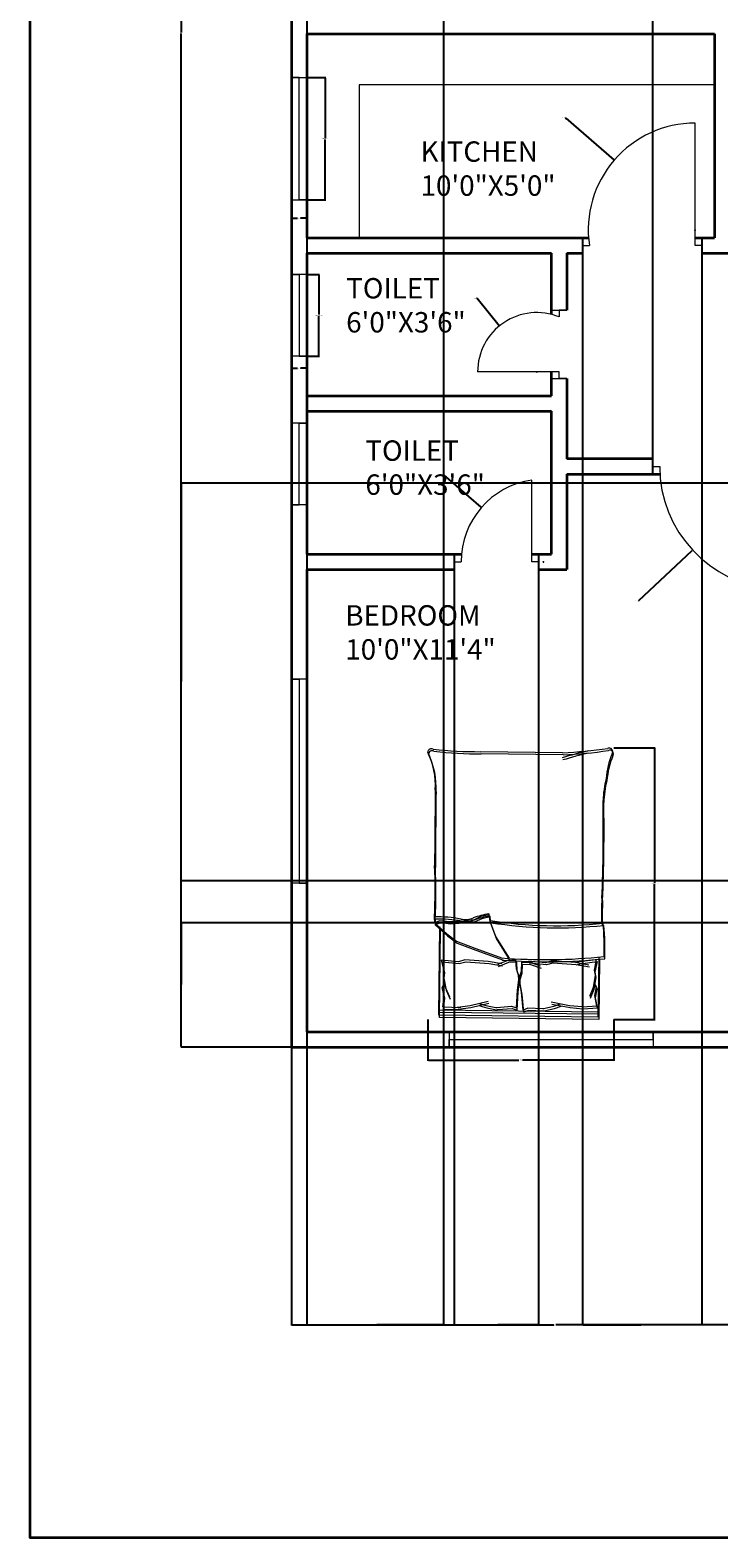
# Model space of a CAD drawing. Units: inches. Extents: x 1721 to 2510, y 1544 to 2360.
# Tile 1 of 10: x 1721 to 1924, y 1544 to 1988. Entities that reach past the tile are written whole.
import ezdxf

# ---------------------------------------------------------------- set-up
doc = ezdxf.new("R2010")
doc.units = ezdxf.units.IN
for name, color, linetype, lineweight in [('A-ANNO-DIMS', 2, 'Continuous', 18), ('A-ANNO-TTLB', 7, 'Continuous', 35), ('A-AREA-IDEN', 7, 'Continuous', 18), ('A-DOOR', 3, 'Continuous', 18), ('A-FLOR-FIXT', 9, 'Continuous', 18), ('A-FURN', 8, 'Continuous', 13), ('A-GLAZ', 4, 'Continuous', 18), ('A-WALL', 7, 'Continuous', 35)]:
    doc.layers.add(name, color=color, linetype=linetype, lineweight=lineweight)
doc.styles.get("Standard").update_dxf_attribs({"font": 'arial.ttf'})
doc.dimstyles.get("Standard").update_dxf_attribs({"dimtxt": 0.18, "dimasz": 0.18, "dimexe": 0.18, "dimexo": 0.0625, "dimgap": 0.09, "dimtad": 0, "dimtih": 1, "dimtoh": 1, "dimdec": 4, "dimzin": 0, "dimdsep": 46, "dimtxsty": 'Standard', "dimcen": 0.09, "dimadec": 0, "dimazin": 0, "dimtfac": 1, "dimtdec": 4, "dimtofl": 0, "dimtmove": 0, "dimatfit": 3, "dimfxl": 1, "dimtolj": 1, "dimtzin": 0, "dimarcsym": 0})

# ---------------------------------------------------------------- blocks, each defined once
blk = doc.blocks.new('BED-DOUBLE')
for p, q in [((39.64, 78.43), (15.52, 78.72)), ((39.64, 78.43), (15.52, 78.72)), ((39.86, 77.8), (15.74, 78.09)), ((39.86, 77.8), (15.74, 78.09)), ((1.93, 30.11), (1.99, 28.4, 3.79)), ((1.93, 30.11), (1.99, 28.4, 3.79)), ((3.5, 28.99), (1.99, 28.4)), ((3.5, 28.99), (1.99, 28.4)), ((1.99, 28.4), (5.58, 25.17)), ((1.99, 28.4), (5.58, 25.17)), ((2.15, 29.48), (2.21, 27.77, 3.79)), ((2.15, 29.48), (2.21, 27.77, 3.79)), ((3.72, 28.36), (2.21, 27.77)), ((3.72, 28.36), (2.21, 27.77)), ((2.21, 27.77), (5.8, 24.54)), ((2.21, 27.77), (5.8, 24.54)), ((3.23, 1.19), (3.55, 27.27)), ((3.23, 1.19), (3.55, 27.27)), ((3.45, 0.56), (3.76, 26.64)), ((3.45, 0.56), (3.76, 26.64)), ((6.54, 28.65), (3.5, 28.99)), ((6.54, 28.65), (3.5, 28.99)), ((6.75, 28.02), (3.72, 28.36)), ((6.75, 28.02), (3.72, 28.36)), ((10.33, 28.91), (6.54, 28.65)), ((10.33, 28.91), (6.54, 28.65)), ((10.55, 28.28), (6.75, 28.02)), ((10.55, 28.28), (6.75, 28.02)), ((13.68, 29.32), (10.33, 28.91)), ((13.68, 29.32), (10.33, 28.91)), ((13.89, 28.69), (10.55, 28.28)), ((13.89, 28.69), (10.55, 28.28)), ((15.66, 30.21), (13.68, 29.32)), ((15.66, 30.21), (13.68, 29.32)), ((15.88, 29.58), (13.89, 28.69)), ((15.88, 29.58), (13.89, 28.69)), ((18.1, 30.79), (15.66, 30.21)), ((18.1, 30.79), (15.66, 30.21)), ((18.31, 30.16), (15.88, 29.58)), ((18.31, 30.16), (15.88, 29.58)), ((18.38, 28.81), (18.1, 30.79)), ((18.38, 28.81), (18.1, 30.79)), ((18.59, 28.18), (18.31, 30.16)), ((18.59, 28.18), (18.31, 30.16)), ((20, 24.39), (18.38, 28.81)), ((20, 24.39), (18.38, 28.81)), ((20.21, 23.76), (18.59, 28.18)), ((20.21, 23.76), (18.59, 28.18)), ((5.58, 25.17), (8.44, 23.01)), ((5.58, 25.17), (8.44, 23.01)), ((5.8, 24.54), (8.66, 22.38)), ((5.8, 24.54), (8.66, 22.38)), ((8.44, 23.01), (13.88, 20.98)), ((8.44, 23.01), (13.88, 20.98)), ((8.66, 22.38), (14.1, 20.35)), ((8.66, 22.38), (14.1, 20.35)), ((24.03, 17.98), (20, 24.39)), ((24.03, 17.98), (20, 24.39)), ((24.24, 17.35), (20.21, 23.76)), ((24.24, 17.35), (20.21, 23.76)), ((13.88, 20.98), (22.02, 18)), ((13.88, 20.98), (22.02, 18)), ((14.1, 20.35), (22.24, 17.37)), ((14.1, 20.35), (22.24, 17.37)), ((50.28, 18.38), (50.07, 0.63)), ((50.28, 18.38), (50.07, 0.63)), ((50.5, 17.75), (50.29, 0)), ((50.5, 17.75), (50.29, 0)), ((9.01, 16.97), (3.98, 17.42)), ((3.98, 17.42), (4.71, 14.34)), ((9.01, 16.97), (3.98, 17.42)), ((3.98, 17.42), (4.71, 14.34)), ((9.23, 16.34), (4.2, 16.8)), ((4.2, 16.8), (4.92, 13.71)), ((9.23, 16.34), (4.2, 16.8)), ((4.2, 16.8), (4.92, 13.71)), ((4.71, 14.34), (4.5, 12.77)), ((4.71, 14.34), (4.5, 12.77)), ((4.92, 13.71), (4.72, 12.14)), ((4.92, 13.71), (4.72, 12.14)), ((10.94, 17.49), (9.01, 16.97)), ((10.94, 17.49), (9.01, 16.97)), ((11.15, 16.86), (9.23, 16.34)), ((11.15, 16.86), (9.23, 16.34)), ((17.8, 16.99), (10.94, 17.49)), ((17.8, 16.99), (10.94, 17.49)), ((18.02, 16.36), (11.15, 16.86)), ((18.02, 16.36), (11.15, 16.86)), ((21.75, 16.29), (17.8, 16.99)), ((21.75, 16.29), (17.8, 16.99)), ((21.96, 15.66), (18.02, 16.36)), ((21.96, 15.66), (18.02, 16.36)), ((23.54, 17.35), (20.51, 16.13)), ((23.54, 17.35), (20.51, 16.13)), ((23.75, 16.73), (20.73, 15.5)), ((23.75, 16.73), (20.73, 15.5)), ((25.94, 17.48), (23.54, 17.35)), ((25.94, 17.48), (23.54, 17.35)), ((26.16, 16.85), (23.75, 16.73)), ((26.16, 16.85), (23.75, 16.73)), ((26.07, 14.85), (25.94, 17.48)), ((26.07, 14.85), (25.94, 17.48)), ((26.73, 13.04), (26.07, 14.85)), ((26.73, 13.04), (26.07, 14.85)), ((26.29, 14.22), (26.16, 16.85)), ((26.29, 14.22), (26.16, 16.85)), ((26.95, 12.41), (26.29, 14.22)), ((26.95, 12.41), (26.29, 14.22)), ((27.02, 12.38), (27.61, 14.21)), ((27.02, 12.38), (27.61, 14.21)), ((27.23, 11.75), (27.82, 13.58)), ((27.23, 11.75), (27.82, 13.58)), ((27.61, 14.21), (27.64, 16.84)), ((27.61, 14.21), (27.64, 16.84)), ((27.64, 16.84), (30.05, 16.81)), ((27.64, 16.84), (30.05, 16.81)), ((27.82, 13.58), (27.85, 16.21)), ((27.82, 13.58), (27.85, 16.21)), ((27.85, 16.21), (30.26, 16.18)), ((27.85, 16.21), (30.26, 16.18)), ((34.67, 16.66), (29.65, 17.12)), ((34.67, 16.66), (29.65, 17.12)), ((34.89, 16.03), (29.86, 16.49)), ((34.89, 16.03), (29.86, 16.49)), ((30.05, 16.81), (33.11, 15.7)), ((30.05, 16.81), (33.11, 15.7)), ((30.26, 16.18), (33.33, 15.07)), ((30.26, 16.18), (33.33, 15.07)), ((36.6, 17.19), (34.67, 16.66)), ((36.6, 17.19), (34.67, 16.66)), ((36.81, 16.56), (34.89, 16.03)), ((36.81, 16.56), (34.89, 16.03)), ((43.46, 16.68), (36.6, 17.19)), ((43.46, 16.68), (36.6, 17.19)), ((43.68, 16.05), (36.81, 16.56)), ((43.68, 16.05), (36.81, 16.56)), ((43.46, 16.68), (44.58, 16.98)), ((43.46, 16.68), (44.58, 16.98)), ((47.41, 15.98), (43.46, 16.68)), ((47.41, 15.98), (43.46, 16.68)), ((43.68, 16.05), (44.79, 16.35)), ((43.68, 16.05), (44.79, 16.35)), ((47.62, 15.35), (43.68, 16.05)), ((47.62, 15.35), (43.68, 16.05)), ((44.58, 16.98), (49.58, 17.63)), ((44.58, 16.98), (49.58, 17.63)), ((44.79, 16.35), (49.8, 17)), ((44.79, 16.35), (49.8, 17)), ((49.58, 17.63), (48.98, 14.52)), ((49.58, 17.63), (48.98, 14.52)), ((48.98, 14.52), (49.24, 12.96)), ((48.98, 14.52), (49.24, 12.96)), ((49.8, 17), (49.19, 13.89)), ((49.8, 17), (49.19, 13.89)), ((49.19, 13.89), (49.46, 12.33)), ((49.19, 13.89), (49.46, 12.33)), ((4.25, 9.35), (4.77, 10.37)), ((4.25, 9.35), (4.77, 10.37)), ((4.8, 6.82), (4.25, 9.35)), ((4.8, 6.82), (4.25, 9.35)), ((4.47, 8.72), (4.98, 9.74)), ((4.47, 8.72), (4.98, 9.74)), ((4.5, 12.77), (5.25, 9.26)), ((4.5, 12.77), (5.25, 9.26)), ((4.72, 12.14), (5.46, 8.63)), ((4.72, 12.14), (5.46, 8.63)), ((5.25, 9.26), (6.37, 6.62)), ((5.25, 9.26), (6.37, 6.62)), ((26.39, 8.62), (26.8, 11.77)), ((26.39, 8.62), (26.8, 11.77)), ((26.61, 7.99), (27.01, 11.14)), ((26.61, 7.99), (27.01, 11.14)), ((26.8, 11.77), (26.73, 13.04)), ((26.8, 11.77), (26.73, 13.04)), ((27.01, 11.14), (26.95, 12.41)), ((27.01, 11.14), (26.95, 12.41)), ((27, 11.1), (27.02, 12.38)), ((27, 11.1), (27.02, 12.38)), ((27.53, 7.98), (27, 11.1)), ((27.53, 7.98), (27, 11.1)), ((27.22, 10.47), (27.23, 11.75)), ((27.22, 10.47), (27.23, 11.75)), ((27.75, 7.35), (27.22, 10.47)), ((27.75, 7.35), (27.22, 10.47)), ((48.63, 9.42), (47.61, 6.74)), ((48.63, 9.42), (47.61, 6.74)), ((49.24, 12.96), (48.63, 9.42)), ((49.24, 12.96), (48.63, 9.42)), ((49.46, 12.33), (48.85, 8.79)), ((49.46, 12.33), (48.85, 8.79)), ((49.63, 9.55), (49.07, 10.55)), ((49.63, 9.55), (49.07, 10.55)), ((49.17, 7.01), (49.63, 9.55)), ((49.17, 7.01), (49.63, 9.55)), ((49.84, 8.92), (49.29, 9.92)), ((49.84, 8.92), (49.29, 9.92)), ((49.39, 6.38), (49.84, 8.92)), ((49.39, 6.38), (49.84, 8.92)), ((4.39, 3.68), (4.8, 6.82)), ((4.39, 3.68), (4.8, 6.82)), ((5.02, 6.19), (4.47, 8.72)), ((5.02, 6.19), (4.47, 8.72)), ((4.61, 3.05), (5.02, 6.19)), ((4.61, 3.05), (5.02, 6.19)), ((5.46, 8.63), (6.59, 5.99)), ((5.46, 8.63), (6.59, 5.99)), ((12.44, 4.09), (17.76, 5.35)), ((12.44, 4.09), (17.76, 5.35)), ((12.65, 3.46), (17.98, 4.72)), ((12.65, 3.46), (17.98, 4.72)), ((15.1, 4.65), (17.12, 4.04)), ((15.1, 4.65), (17.12, 4.04)), ((26.09, 3.36), (26.39, 8.62)), ((26.09, 3.36), (26.39, 8.62)), ((26.3, 2.73), (26.61, 7.99)), ((26.3, 2.73), (26.61, 7.99)), ((28.04, 2.73), (27.53, 7.98)), ((28.04, 2.73), (27.53, 7.98)), ((28.25, 2.1), (27.75, 7.35)), ((28.25, 2.1), (27.75, 7.35)), ((41.65, 3.98), (36.28, 5.04)), ((41.65, 3.98), (36.28, 5.04)), ((38.96, 4.44), (36.97, 3.75)), ((38.96, 4.44), (36.97, 3.75)), ((48.85, 8.79), (47.82, 6.11)), ((48.85, 8.79), (47.82, 6.11)), ((49.7, 3.88), (49.17, 7.01)), ((49.7, 3.88), (49.17, 7.01)), ((49.92, 3.25), (49.39, 6.38)), ((49.92, 3.25), (49.39, 6.38)), ((50.07, 0.63), (3.23, 1.19)), ((50.07, 0.63), (3.23, 1.19)), ((50.09, 2.13), (3.25, 2.69)), ((50.09, 2.13), (3.25, 2.69)), ((50.29, 0), (3.45, 0.56)), ((50.29, 0), (3.45, 0.56)), ((50.31, 1.5), (3.47, 2.06)), ((50.31, 1.5), (3.47, 2.06)), ((4.39, 3.68), (9.69, 3.52)), ((4.39, 3.68), (9.69, 3.52)), ((4.61, 3.05), (9.9, 2.89)), ((4.61, 3.05), (9.9, 2.89)), ((8.71, 3.62), (12.44, 4.09)), ((8.71, 3.62), (12.44, 4.09)), ((9.69, 3.52), (8.71, 3.62)), ((9.69, 3.52), (8.71, 3.62)), ((8.92, 2.99), (12.65, 3.46)), ((8.92, 2.99), (12.65, 3.46)), ((9.9, 2.89), (8.92, 2.99)), ((9.9, 2.89), (8.92, 2.99)), ((15.32, 4.02), (17.34, 3.41)), ((15.32, 4.02), (17.34, 3.41)), ((17.12, 4.04), (19.98, 3.48)), ((17.12, 4.04), (19.98, 3.48)), ((17.34, 3.41), (20.2, 2.85)), ((17.34, 3.41), (20.2, 2.85)), ((19.98, 3.48), (20.3, 3.49)), ((19.98, 3.48), (20.3, 3.49)), ((20.2, 2.85), (20.52, 2.86)), ((20.2, 2.85), (20.52, 2.86)), ((20.3, 3.49), (24.64, 3.85)), ((20.3, 3.49), (24.64, 3.85)), ((20.52, 2.86), (24.86, 3.22)), ((20.52, 2.86), (24.86, 3.22)), ((24.64, 3.85), (26.09, 3.36)), ((24.64, 3.85), (26.09, 3.36)), ((24.86, 3.22), (26.3, 2.73)), ((24.86, 3.22), (26.3, 2.73)), ((29.46, 3.28), (28.04, 2.73)), ((29.46, 3.28), (28.04, 2.73)), ((29.68, 2.65), (28.25, 2.1)), ((29.68, 2.65), (28.25, 2.1)), ((33.81, 3.08), (29.46, 3.28)), ((33.81, 3.08), (29.46, 3.28)), ((34.03, 2.45), (29.68, 2.65)), ((34.03, 2.45), (29.68, 2.65)), ((34.13, 3.08), (33.81, 3.08)), ((34.13, 3.08), (33.81, 3.08)), ((34.35, 2.45), (34.03, 2.45)), ((34.35, 2.45), (34.03, 2.45)), ((36.97, 3.75), (34.13, 3.08)), ((36.97, 3.75), (34.13, 3.08)), ((37.19, 3.12), (34.35, 2.45)), ((37.19, 3.12), (34.35, 2.45)), ((41.87, 3.35), (36.49, 4.41)), ((41.87, 3.35), (36.49, 4.41)), ((39.18, 3.81), (37.19, 3.12)), ((39.18, 3.81), (37.19, 3.12)), ((45.39, 3.65), (41.65, 3.98)), ((45.39, 3.65), (41.65, 3.98)), ((45.61, 3.02), (41.87, 3.35)), ((45.61, 3.02), (41.87, 3.35)), ((45.5, 3.63), (45.39, 3.65)), ((45.5, 3.63), (45.39, 3.65)), ((49.7, 3.91), (45.5, 3.63)), ((49.7, 3.91), (45.5, 3.63)), ((45.71, 3), (45.61, 3.02)), ((45.71, 3), (45.61, 3.02)), ((49.91, 3.28), (45.71, 3)), ((49.91, 3.28), (45.71, 3))]:
    blk.add_line(p, q)
for centre, radius, start, end in [((1.08, 78.52), 1.08, 61.9736, 175.3348), ((1.08, 78.52), 1.08, 61.9736, 175.3348), ((-20.36, 68.78), 22.61, 356.7862, 25.7829), ((-20.36, 68.78), 22.61, 356.7862, 25.7829), ((1.29, 77.89), 1.08, 61.9736, 175.3348), ((1.29, 77.89), 1.08, 61.9736, 175.3348), ((-20.14, 68.15), 22.61, 356.7862, 25.7829), ((-20.14, 68.15), 22.61, 356.7862, 25.7829), ((15.63, 209.12), 130.4, 263.8146, 269.9499), ((15.63, 209.12), 130.4, 263.8146, 269.9499), ((15.85, 208.49), 130.4, 263.8146, 269.9499), ((15.85, 208.49), 130.4, 263.8146, 269.9499), ((70.08, -22.85), 104.34, 102.698, 107.0202), ((70.08, -22.85), 104.34, 102.698, 107.0202), ((34.83, 197.67), 119.34, 272.3106, 278.7239), ((34.83, 197.67), 119.34, 272.3106, 278.7239), ((70.29, -23.48), 104.34, 102.698, 107.0202), ((70.29, -23.48), 104.34, 102.698, 107.0202), ((35.05, 197.04), 119.34, 272.3106, 278.7239), ((35.05, 197.04), 119.34, 272.3106, 278.7239), ((75.53, 69.21), 23.09, 157.2899, 175.9668), ((75.53, 69.21), 23.09, 157.2899, 175.9668), ((75.75, 68.58), 23.09, 157.2899, 175.9668), ((75.75, 68.58), 23.09, 157.2899, 175.9668), ((53.35, 78.73), 1.07, 325.4884, 112.793), ((53.35, 78.73), 1.07, 325.4884, 112.793), ((53.56, 78.1), 1.07, 325.4884, 112.793), ((53.56, 78.1), 1.07, 325.4884, 112.793), ((4473.12, 14.21), 4471.22, 179.317, 179.60172), ((4473.12, 14.21), 4471.22, 179.317, 179.60172), ((4473.34, 13.58), 4471.22, 179.317, 179.60172), ((4473.34, 13.58), 4471.22, 179.317, 179.60172), ((80.6, 63.5), 29.05, 165.3797, 178.2261), ((80.6, 63.5), 29.05, 165.3797, 178.2261), ((80.81, 62.87), 29.05, 165.3797, 178.2261), ((80.81, 62.87), 29.05, 165.3797, 178.2261), ((-421.08, 55.88), 472.73, 357.5425, 1.0334), ((-421.08, 55.88), 472.73, 357.5425, 1.0334), ((-420.87, 55.25), 472.73, 357.5425, 1.0334), ((-420.87, 55.25), 472.73, 357.5425, 1.0334), ((-124.73, 38.32), 126.93, 356.294, 3.1513), ((-124.73, 38.32), 126.93, 356.294, 3.1513), ((-124.51, 37.69), 126.93, 356.294, 3.1513), ((-124.51, 37.69), 126.93, 356.294, 3.1513), ((217.81, 29.18), 166.73, 177.791, 180.323), ((217.81, 29.18), 166.73, 177.791, 180.323), ((218.03, 28.55), 166.73, 177.791, 180.323), ((218.03, 28.55), 166.73, 177.791, 180.323), ((3.1, -5.33), 35.46, 79.1911, 91.8805), ((3.1, -5.33), 35.46, 79.1911, 91.8805), ((3.31, -5.96), 35.46, 79.1911, 91.8805), ((3.31, -5.96), 35.46, 79.1911, 91.8805), ((11.02, 35.47), 6.1, 257.9756, 293.0532), ((11.02, 35.47), 6.1, 257.9756, 293.0532), ((11.23, 34.84), 6.1, 257.9756, 293.0532), ((11.23, 34.84), 6.1, 257.9756, 293.0532), ((22.96, 2.41), 29.06, 99.9765, 109.1954), ((22.96, 2.41), 29.06, 99.9765, 109.1954), ((23.18, 1.78), 29.06, 99.9765, 109.1954), ((23.18, 1.78), 29.06, 99.9765, 109.1954), ((17.93, 30.85), 0.181, 339.5612, 90.4525), ((17.93, 30.85), 0.181, 339.5612, 90.4525), ((18.15, 30.22), 0.181, 339.5612, 90.4525), ((18.15, 30.22), 0.181, 339.5612, 90.4525), ((37.91, 154), 126.46, 261.0993, 276.2154), ((37.91, 154), 126.46, 261.0993, 276.2154), ((38.12, 153.37), 126.46, 261.0993, 276.2154), ((38.12, 153.37), 126.46, 261.0993, 276.2154), ((-29.75, 21.28), 81.65, 358.0366, 4.9188), ((-29.75, 21.28), 81.65, 358.0366, 4.9188), ((-29.53, 20.65), 81.65, 358.0366, 4.9188), ((-29.53, 20.65), 81.65, 358.0366, 4.9188), ((34.68, 179.26), 161.69, 265.4014, 276.097), ((34.68, 179.26), 161.69, 265.4014, 276.097), ((34.89, 178.63), 161.69, 265.4014, 276.097), ((34.89, 178.63), 161.69, 265.4014, 276.097)]:
    blk.add_arc(centre, radius, start, end)
blk = doc.blocks.new('WIN-60IN-A')
for p, q in [((4.5, 60), (0, 60)), ((2.25, 0), (2.25, 60)), ((2.25, 60), (4.5, 60)), ((4.5, 0), (0, 0)), ((0, 0), (2.25, 0))]:
    blk.add_line(p, q)
blk = doc.blocks.new('WIN-24IN-A')
for p, q in [((4.5, 24), (0, 24)), ((0, 24), (2.25, 24)), ((2.25, 24), (2.25, 0)), ((4.5, 0), (0, 0)), ((2.25, 0), (4.5, 0))]:
    blk.add_line(p, q)
blk = doc.blocks.new('WIN-36IN-A')
for p, q in [((2.25, 36), (0, 36)), ((0, 36), (4.5, 36)), ((2.25, 0), (2.25, 36)), ((0, 0), (4.5, 0)), ((4.5, 0), (2.25, 0))]:
    blk.add_line(p, q)
blk = doc.blocks.new('*D14')
at = {"layer": 'A-ANNO-DIMS', "color": 0, "lineweight": -2, "transparency": 16777216}
for p, q in [((1892.88, 1776.68), (1904.98, 1776.68)), ((1904.8, 1776.5), (1904.8, 1736.91)), ((1904.8, 1696.96), (1904.8, 1736.55)), ((1892.88, 1696.78), (1904.98, 1696.78))]:
    blk.add_line(p, q, dxfattribs=at)
at = {"layer": 'A-ANNO-DIMS', "color": 0, "transparency": 16777216}
for points in [[(1904.77, 1776.5), (1904.83, 1776.5), (1904.8, 1776.68)], [(1904.77, 1696.96), (1904.83, 1696.96), (1904.8, 1696.78)]]:
    blk.add_solid(points, dxfattribs=at)
at = {"layer": 'Defpoints', "color": 0, "transparency": 16777216}
for p in [(1892.81, 1776.68), (1904.8, 1776.68), (1892.81, 1696.78)]:
    blk.add_point(p, dxfattribs=at)
at = {"layer": 'A-ANNO-DIMS', "color": 0, "transparency": 16777216, "insert": (1904.8, 1736.73), "char_height": 0.18, "attachment_point": 5}
blk.add_mtext('\\A1;DOUBLE BED 80 TYP.', dxfattribs=at)
blk = doc.blocks.new('*D15')
at = {"layer": 'A-ANNO-DIMS', "color": 0, "lineweight": -2, "transparency": 16777216}
for p, q in [((1838.1, 1696.72), (1838.1, 1684.62)), ((1892.81, 1696.72), (1892.81, 1684.62)), ((1838.28, 1684.8), (1864.93, 1684.8)), ((1892.63, 1684.8), (1865.99, 1684.8))]:
    blk.add_line(p, q, dxfattribs=at)
at = {"layer": 'A-ANNO-DIMS', "color": 0, "transparency": 16777216}
for points in [[(1838.28, 1684.83), (1838.28, 1684.77), (1838.1, 1684.8)], [(1892.63, 1684.83), (1892.63, 1684.77), (1892.81, 1684.8)]]:
    blk.add_solid(points, dxfattribs=at)
at = {"layer": 'Defpoints', "color": 0, "transparency": 16777216}
for p in [(1838.1, 1696.78), (1892.81, 1696.78), (1892.81, 1684.8)]:
    blk.add_point(p, dxfattribs=at)
at = {"layer": 'A-ANNO-DIMS', "color": 0, "transparency": 16777216, "insert": (1865.46, 1684.8), "char_height": 0.18, "attachment_point": 5}
blk.add_mtext('\\A1;55 TYP.', dxfattribs=at)
blk = doc.blocks.new('*D22')
at = {"layer": 'A-ANNO-DIMS', "color": 0, "lineweight": -2, "transparency": 16777216}
for p, q in [((1802.56, 1973.78), (1808.08, 1973.78)), ((1807.9, 1973.6), (1807.9, 1955.97)), ((1807.9, 1937.96), (1807.9, 1955.6)), ((1802.56, 1937.78), (1808.08, 1937.78))]:
    blk.add_line(p, q, dxfattribs=at)
at = {"layer": 'A-ANNO-DIMS', "color": 0, "transparency": 16777216}
for points in [[(1807.87, 1973.6), (1807.93, 1973.6), (1807.9, 1973.78)], [(1807.87, 1937.96), (1807.93, 1937.96), (1807.9, 1937.78)]]:
    blk.add_solid(points, dxfattribs=at)
at = {"layer": 'Defpoints', "color": 0, "transparency": 16777216}
for p in [(1802.5, 1973.78), (1807.9, 1973.78), (1802.5, 1937.78)]:
    blk.add_point(p, dxfattribs=at)
at = {"layer": 'A-ANNO-DIMS', "color": 0, "transparency": 16777216, "insert": (1807.9, 1955.78), "char_height": 0.18, "attachment_point": 5}
blk.add_mtext('\\A1;WINDOW A 36 TYP.', dxfattribs=at)
blk = doc.blocks.new('*D23')
at = {"layer": 'A-ANNO-DIMS', "color": 0, "lineweight": -2, "transparency": 16777216}
for p, q in [((1798, 1937.72), (1798, 1932.2)), ((1802.5, 1937.72), (1802.5, 1932.2)), ((1798.18, 1932.38), (1799.79, 1932.38)), ((1802.32, 1932.38), (1800.71, 1932.38))]:
    blk.add_line(p, q, dxfattribs=at)
at = {"layer": 'A-ANNO-DIMS', "color": 0, "transparency": 16777216}
for points in [[(1798.18, 1932.41), (1798.18, 1932.35), (1798, 1932.38)], [(1802.32, 1932.41), (1802.32, 1932.35), (1802.5, 1932.38)]]:
    blk.add_solid(points, dxfattribs=at)
at = {"layer": 'Defpoints', "color": 0, "transparency": 16777216}
for p in [(1798, 1937.78), (1802.5, 1937.78), (1802.5, 1932.38)]:
    blk.add_point(p, dxfattribs=at)
at = {"layer": 'A-ANNO-DIMS', "color": 0, "transparency": 16777216, "insert": (1800.25, 1932.38), "char_height": 0.18, "attachment_point": 5}
blk.add_mtext('\\A1;5 TYP.', dxfattribs=at)
blk = doc.blocks.new('*D26')
at = {"layer": 'A-ANNO-DIMS', "color": 0, "lineweight": -2, "transparency": 16777216}
for p, q in [((1802.56, 1915.87), (1806.28, 1915.87)), ((1806.1, 1915.69), (1806.1, 1904.05)), ((1806.1, 1892.05), (1806.1, 1903.68)), ((1802.56, 1891.87), (1806.28, 1891.87))]:
    blk.add_line(p, q, dxfattribs=at)
at = {"layer": 'A-ANNO-DIMS', "color": 0, "transparency": 16777216}
for points in [[(1806.07, 1915.69), (1806.13, 1915.69), (1806.1, 1915.87)], [(1806.07, 1892.05), (1806.13, 1892.05), (1806.1, 1891.87)]]:
    blk.add_solid(points, dxfattribs=at)
at = {"layer": 'Defpoints', "color": 0, "transparency": 16777216}
for p in [(1802.5, 1915.87), (1806.1, 1915.87), (1802.5, 1891.87)]:
    blk.add_point(p, dxfattribs=at)
at = {"layer": 'A-ANNO-DIMS', "color": 0, "transparency": 16777216, "insert": (1806.1, 1903.87), "char_height": 0.18, "attachment_point": 5}
blk.add_mtext('\\A1;WINDOW A 24 TYP.', dxfattribs=at)
blk = doc.blocks.new('*D27')
at = {"layer": 'A-ANNO-DIMS', "color": 0, "lineweight": -2, "transparency": 16777216}
for p, q in [((1798, 1891.8), (1798, 1888.09)), ((1802.5, 1891.8), (1802.5, 1888.09)), ((1798.18, 1888.27), (1799.79, 1888.27)), ((1802.32, 1888.27), (1800.71, 1888.27))]:
    blk.add_line(p, q, dxfattribs=at)
at = {"layer": 'A-ANNO-DIMS', "color": 0, "transparency": 16777216}
for points in [[(1798.18, 1888.3), (1798.18, 1888.24), (1798, 1888.27)], [(1802.32, 1888.3), (1802.32, 1888.24), (1802.5, 1888.27)]]:
    blk.add_solid(points, dxfattribs=at)
at = {"layer": 'Defpoints', "color": 0, "transparency": 16777216}
for p in [(1798, 1891.87), (1802.5, 1891.87), (1802.5, 1888.27)]:
    blk.add_point(p, dxfattribs=at)
at = {"layer": 'A-ANNO-DIMS', "color": 0, "transparency": 16777216, "insert": (1800.25, 1888.27), "char_height": 0.18, "attachment_point": 5}
blk.add_mtext('\\A1;5 TYP.', dxfattribs=at)
blk = doc.blocks.new('*D41')
at = {"layer": 'A-ANNO-DIMS', "color": 0, "lineweight": -2, "transparency": 16777216}
for p, q in [((1797.94, 2285.13), (1765.42, 2285.13)), ((1765.6, 2284.95), (1765.6, 1987.06)), ((1765.6, 1688.81), (1765.6, 1986.7)), ((1797.94, 1688.63), (1765.42, 1688.63))]:
    blk.add_line(p, q, dxfattribs=at)
at = {"layer": 'A-ANNO-DIMS', "color": 0, "transparency": 16777216}
for points in [[(1765.57, 2284.95), (1765.63, 2284.95), (1765.6, 2285.13)], [(1765.57, 1688.81), (1765.63, 1688.81), (1765.6, 1688.63)]]:
    blk.add_solid(points, dxfattribs=at)
at = {"layer": 'Defpoints', "color": 0, "transparency": 16777216}
for p in [(1765.6, 2285.13), (1798, 2285.13), (1798, 1688.63)]:
    blk.add_point(p, dxfattribs=at)
at = {"layer": 'A-ANNO-DIMS', "color": 0, "transparency": 16777216, "insert": (1765.6, 1986.88), "char_height": 0.18, "attachment_point": 5}
blk.add_mtext('\\A1;596.5', dxfattribs=at)
blk = doc.blocks.new('*D42')
at = {"layer": 'A-ANNO-DIMS', "color": 0, "lineweight": -2, "transparency": 16777216}
for p, q in [((1798, 1688.57), (1798, 1606.75)), ((1953, 1688.57), (1953, 1606.75)), ((1798.18, 1606.93), (1875.22, 1606.93)), ((1952.82, 1606.93), (1875.78, 1606.93))]:
    blk.add_line(p, q, dxfattribs=at)
at = {"layer": 'A-ANNO-DIMS', "color": 0, "transparency": 16777216}
for points in [[(1798.18, 1606.96), (1798.18, 1606.9), (1798, 1606.93)], [(1952.82, 1606.96), (1952.82, 1606.9), (1953, 1606.93)]]:
    blk.add_solid(points, dxfattribs=at)
at = {"layer": 'Defpoints', "color": 0, "transparency": 16777216}
for p in [(1798, 1688.63), (1953, 1688.63), (1953, 1606.93)]:
    blk.add_point(p, dxfattribs=at)
at = {"layer": 'A-ANNO-DIMS', "color": 0, "transparency": 16777216, "insert": (1875.5, 1606.93), "char_height": 0.18, "attachment_point": 5}
blk.add_mtext('\\A1;155', dxfattribs=at)
blk = doc.blocks.new('*D53')
at = {"layer": 'A-ANNO-DIMS', "color": 0, "lineweight": -2, "transparency": 16777216}
for p, q in [((2127.44, 1854.49), (1765.42, 1854.49)), ((1765.6, 1854.31), (1765.6, 1796.17)), ((1765.6, 1737.67), (1765.6, 1795.81)), ((2127.44, 1737.49), (1765.42, 1737.49))]:
    blk.add_line(p, q, dxfattribs=at)
at = {"layer": 'A-ANNO-DIMS', "color": 0, "transparency": 16777216}
for points in [[(1765.57, 1854.31), (1765.63, 1854.31), (1765.6, 1854.49)], [(1765.57, 1737.67), (1765.63, 1737.67), (1765.6, 1737.49)]]:
    blk.add_solid(points, dxfattribs=at)
at = {"layer": 'Defpoints', "color": 0, "transparency": 16777216}
for p in [(1765.6, 1854.49), (2127.5, 1854.49), (2127.5, 1737.49)]:
    blk.add_point(p, dxfattribs=at)
at = {"layer": 'A-ANNO-DIMS', "color": 0, "transparency": 16777216, "insert": (1765.6, 1795.99), "char_height": 0.18, "attachment_point": 5}
blk.add_mtext('\\A1;117', dxfattribs=at)
blk = doc.blocks.new('*D56')
at = {"layer": 'A-ANNO-DIMS', "color": 0, "lineweight": -2, "transparency": 16777216}
for p, q in [((1802.5, 2280.57), (1802.5, 1606.75)), ((1842.73, 2280.57), (1842.73, 1606.75)), ((1802.68, 1606.93), (1822.15, 1606.93)), ((1842.55, 1606.93), (1823.08, 1606.93))]:
    blk.add_line(p, q, dxfattribs=at)
at = {"layer": 'A-ANNO-DIMS', "color": 0, "transparency": 16777216}
for points in [[(1802.68, 1606.96), (1802.68, 1606.9), (1802.5, 1606.93)], [(1842.55, 1606.96), (1842.55, 1606.9), (1842.73, 1606.93)]]:
    blk.add_solid(points, dxfattribs=at)
at = {"layer": 'Defpoints', "color": 0, "transparency": 16777216}
for p in [(1802.5, 2280.63), (1842.73, 2280.63), (1842.73, 1606.93)]:
    blk.add_point(p, dxfattribs=at)
at = {"layer": 'A-ANNO-DIMS', "color": 0, "transparency": 16777216, "insert": (1822.61, 1606.93), "char_height": 0.18, "attachment_point": 5}
blk.add_mtext('\\A1;40.224', dxfattribs=at)
blk = doc.blocks.new('*D59')
at = {"layer": 'A-ANNO-DIMS', "color": 0, "lineweight": -2, "transparency": 16777216}
for p, q in [((1904.34, 1857.19), (1904.34, 2317.71)), ((1904.52, 2317.53), (1921.76, 2317.53)), ((1939.78, 2317.53), (1922.54, 2317.53)), ((1939.96, 1857.19), (1939.96, 2317.71))]:
    blk.add_line(p, q, dxfattribs=at)
at = {"layer": 'A-ANNO-DIMS', "color": 0, "transparency": 16777216}
for points in [[(1904.52, 2317.56), (1904.52, 2317.5), (1904.34, 2317.53)], [(1939.78, 2317.56), (1939.78, 2317.5), (1939.96, 2317.53)]]:
    blk.add_solid(points, dxfattribs=at)
at = {"layer": 'Defpoints', "color": 0, "transparency": 16777216}
for p in [(1939.96, 2317.53), (1904.34, 1857.13), (1939.96, 1857.13)]:
    blk.add_point(p, dxfattribs=at)
at = {"layer": 'A-ANNO-DIMS', "color": 0, "transparency": 16777216, "insert": (1922.15, 2317.53), "char_height": 0.18, "attachment_point": 5}
blk.add_mtext('\\A1;35.62', dxfattribs=at)
blk = doc.blocks.new('*D60')
at = {"layer": 'A-ANNO-DIMS', "color": 0, "lineweight": -2, "transparency": 16777216}
for p, q in [((1883.64, 1926.57), (1883.64, 1606.75)), ((1918.77, 1926.57), (1918.77, 1606.75)), ((1883.82, 1606.93), (1900.74, 1606.93)), ((1918.59, 1606.93), (1901.67, 1606.93))]:
    blk.add_line(p, q, dxfattribs=at)
at = {"layer": 'A-ANNO-DIMS', "color": 0, "transparency": 16777216}
for points in [[(1883.82, 1606.96), (1883.82, 1606.9), (1883.64, 1606.93)], [(1918.59, 1606.96), (1918.59, 1606.9), (1918.77, 1606.93)]]:
    blk.add_solid(points, dxfattribs=at)
at = {"layer": 'Defpoints', "color": 0, "transparency": 16777216}
for p in [(1883.64, 1926.63), (1918.77, 1926.63), (1918.77, 1606.93)]:
    blk.add_point(p, dxfattribs=at)
at = {"layer": 'A-ANNO-DIMS', "color": 0, "transparency": 16777216, "insert": (1901.21, 1606.93), "char_height": 0.18, "attachment_point": 5}
blk.add_mtext('\\A1;35.134', dxfattribs=at)
blk = doc.blocks.new('*D61')
at = {"layer": 'A-ANNO-DIMS', "color": 0, "lineweight": -2, "transparency": 16777216}
for p, q in [((1845.9, 1833.57), (1845.9, 1606.75)), ((1870.71, 1833.57), (1870.71, 1606.75)), ((1846.08, 1606.93), (1857.93, 1606.93)), ((1870.53, 1606.93), (1858.69, 1606.93))]:
    blk.add_line(p, q, dxfattribs=at)
at = {"layer": 'A-ANNO-DIMS', "color": 0, "transparency": 16777216}
for points in [[(1846.08, 1606.96), (1846.08, 1606.9), (1845.9, 1606.93)], [(1870.53, 1606.96), (1870.53, 1606.9), (1870.71, 1606.93)]]:
    blk.add_solid(points, dxfattribs=at)
at = {"layer": 'Defpoints', "color": 0, "transparency": 16777216}
for p in [(1845.9, 1833.63), (1870.71, 1833.63), (1870.71, 1606.93)]:
    blk.add_point(p, dxfattribs=at)
at = {"layer": 'A-ANNO-DIMS', "color": 0, "transparency": 16777216, "insert": (1858.31, 1606.93), "char_height": 0.18, "attachment_point": 5}
blk.add_mtext('\\A1;24.81', dxfattribs=at)
blk = doc.blocks.new('*D67')
at = {"layer": 'A-ANNO-DIMS', "color": 0, "lineweight": -2, "transparency": 16777216}
for p, q in [((2042.44, 1725.13), (1765.42, 1725.13)), ((1765.6, 1724.95), (1765.6, 1707.06)), ((1765.6, 1688.81), (1765.6, 1706.7)), ((2042.44, 1688.63), (1765.42, 1688.63))]:
    blk.add_line(p, q, dxfattribs=at)
at = {"layer": 'A-ANNO-DIMS', "color": 0, "transparency": 16777216}
for points in [[(1765.57, 1724.95), (1765.63, 1724.95), (1765.6, 1725.13)], [(1765.57, 1688.81), (1765.63, 1688.81), (1765.6, 1688.63)]]:
    blk.add_solid(points, dxfattribs=at)
at = {"layer": 'Defpoints', "color": 0, "transparency": 16777216}
for p in [(1765.6, 1725.13), (2042.5, 1725.13), (2042.5, 1688.63)]:
    blk.add_point(p, dxfattribs=at)
at = {"layer": 'A-ANNO-DIMS', "color": 0, "transparency": 16777216, "insert": (1765.6, 1706.88), "char_height": 0.18, "attachment_point": 5}
blk.add_mtext('\\A1;36.5', dxfattribs=at)
blk = doc.blocks.new('*D73')
at = {"layer": 'A-ANNO-DIMS', "color": 0, "lineweight": -2, "transparency": 16777216}
for p, q in [((1942.33, 1859.38), (1942.51, 1859.38)), ((1942.42, 1859.29), (1942.42, 1859.47)), ((1900.23, 1819.97), (1915.92, 1834.63)), ((1900.05, 1819.97), (1900.23, 1819.97))]:
    blk.add_line(p, q, dxfattribs=at)
at = {"layer": 'A-ANNO-DIMS', "color": 0, "transparency": 16777216}
blk.add_solid([(1915.9, 1834.65), (1915.94, 1834.61), (1916.05, 1834.75)], dxfattribs=at)
at = {"layer": 'Defpoints', "color": 0, "transparency": 16777216}
for p in [(1942.42, 1859.38), (1916.05, 1834.75)]:
    blk.add_point(p, dxfattribs=at)
at = {"layer": 'A-ANNO-DIMS', "color": 0, "transparency": 16777216, "insert": (1899.5, 1819.97), "char_height": 0.18, "attachment_point": 5}
blk.add_mtext('\\A1;R36.084', dxfattribs=at)
blk = doc.blocks.new('*D75')
at = {"layer": 'A-ANNO-DIMS', "color": 0, "lineweight": -2, "transparency": 16777216}
for p, q in [((1878.52, 1961.85), (1878.7, 1961.85)), ((1878.7, 1961.85), (1892.84, 1949.62)), ((1916.68, 1928.92), (1916.86, 1928.92)), ((1916.77, 1928.83), (1916.77, 1929.01))]:
    blk.add_line(p, q, dxfattribs=at)
at = {"layer": 'A-ANNO-DIMS', "color": 0, "transparency": 16777216}
blk.add_solid([(1892.86, 1949.64), (1892.82, 1949.59), (1892.98, 1949.5)], dxfattribs=at)
at = {"layer": 'Defpoints', "color": 0, "transparency": 16777216}
for p in [(1892.98, 1949.5), (1916.77, 1928.92)]:
    blk.add_point(p, dxfattribs=at)
at = {"layer": 'A-ANNO-DIMS', "color": 0, "transparency": 16777216, "insert": (1878.04, 1961.85), "char_height": 0.18, "attachment_point": 5}
blk.add_mtext('\\A1;R31.46', dxfattribs=at)
blk = doc.blocks.new('*D83')
at = {"layer": 'A-ANNO-DIMS', "color": 0, "lineweight": -2, "transparency": 16777216}
for p, q in [((1842.66, 1856.79), (1842.84, 1856.79)), ((1842.84, 1856.79), (1853.69, 1847.38)), ((1872.06, 1831.38), (1872.24, 1831.38)), ((1872.15, 1831.29), (1872.15, 1831.47))]:
    blk.add_line(p, q, dxfattribs=at)
at = {"layer": 'A-ANNO-DIMS', "color": 0, "transparency": 16777216}
blk.add_solid([(1853.71, 1847.4), (1853.67, 1847.36), (1853.83, 1847.26)], dxfattribs=at)
at = {"layer": 'Defpoints', "color": 0, "transparency": 16777216}
for p in [(1853.83, 1847.26), (1872.15, 1831.38)]:
    blk.add_point(p, dxfattribs=at)
at = {"layer": 'A-ANNO-DIMS', "color": 0, "transparency": 16777216, "insert": (1842.11, 1856.79), "char_height": 0.18, "attachment_point": 5}
blk.add_mtext('\\A1;R24.244', dxfattribs=at)
blk = doc.blocks.new('*D91')
at = {"layer": 'A-ANNO-DIMS', "color": 0, "lineweight": -2, "transparency": 16777216}
for p, q in [((1852.43, 1908.87), (1852.61, 1908.87)), ((1852.61, 1908.87), (1859.09, 1900.89)), ((1870.09, 1887.22), (1870.27, 1887.22)), ((1870.18, 1887.13), (1870.18, 1887.31))]:
    blk.add_line(p, q, dxfattribs=at)
at = {"layer": 'A-ANNO-DIMS', "color": 0, "transparency": 16777216}
blk.add_solid([(1859.11, 1900.91), (1859.07, 1900.87), (1859.2, 1900.75)], dxfattribs=at)
at = {"layer": 'Defpoints', "color": 0, "transparency": 16777216}
for p in [(1859.2, 1900.75), (1870.18, 1887.22)]:
    blk.add_point(p, dxfattribs=at)
at = {"layer": 'A-ANNO-DIMS', "color": 0, "transparency": 16777216, "insert": (1851.95, 1908.87), "char_height": 0.18, "attachment_point": 5}
blk.add_mtext('\\A1;R17.43', dxfattribs=at)

msp = doc.modelspace()

# ---------------------------------------------------------------- linework, layer by layer
at = {"layer": 'A-ANNO-TTLB'}
msp.add_lwpolyline([(1721.1268, 2360.2177), (2509.707, 2360.2177), (2509.707, 1544.3037), (1721.1268, 1544.3037)], close=True, dxfattribs=at)
at = {"layer": 'A-DOOR'}
for p, q in [((1916.7745, 1924.3798), (1916.7745, 1960.3798)), ((1883.6405, 1926.6298), (1883.6405, 1922.1298)), ((1918.7745, 1926.6298), (1918.7745, 1922.1298)), ((1883.6405, 1922.1298), (1883.6405, 1924.3798)), ((1883.6405, 1924.3798), (1885.6405, 1924.3798)), ((1918.7745, 1924.3798), (1916.7745, 1924.3798)), ((1918.7745, 1922.1298), (1918.7745, 1924.3798)), ((1874.5024, 1905.3589), (1879.0024, 1905.3589)), ((1879.0024, 1905.3589), (1876.7524, 1905.3589)), ((1876.7524, 1905.3589), (1876.7524, 1903.3589)), ((1876.7524, 1887.2154), (1852.7524, 1887.2154)), ((1874.5024, 1885.2154), (1879.0024, 1885.2154)), ((1876.7524, 1885.2154), (1876.7524, 1887.2154)), ((1879.0024, 1885.2154), (1876.7524, 1885.2154)), ((1904.3387, 1861.6298), (1904.3387, 1857.1298)), ((1904.3387, 1857.1298), (1904.3387, 1859.3798)), ((1904.3387, 1859.3798), (1906.3387, 1859.3798)), ((1868.7144, 1831.3798), (1868.7144, 1855.3798)), ((1845.9031, 1833.6298), (1845.9031, 1833.6298)), ((1845.9031, 1833.6298), (1845.9031, 1829.1298)), ((1845.9031, 1829.1298), (1845.9031, 1831.3798)), ((1845.9031, 1831.3798), (1847.9031, 1831.3798)), ((1870.7144, 1831.3798), (1868.7144, 1831.3798)), ((1870.7144, 1833.6298), (1870.7144, 1829.1298)), ((1870.7144, 1829.1298), (1870.7144, 1831.3798))]:
    msp.add_line(p, q, dxfattribs=at)
for centre, radius, start, end in [((1916.7745, 1928.917), 31.4628, 90, 188.291452), ((1870.1818, 1887.2154), 17.4294, 67.853108, 180), ((1942.4229, 1859.3798), 36.0842, 180, 266.085268), ((1872.1473, 1831.3798), 24.2443, 98.140338, 180)]:
    msp.add_arc(centre, radius, start, end, dxfattribs=at)
at = {"layer": 'A-FLOR-FIXT'}
for p, q in [((1922.5024, 1971.599), (1817.8821, 1971.599)), ((1817.8821, 1971.599), (1817.8821, 1926.6298))]:
    msp.add_line(p, q, dxfattribs=at)
at = {"layer": 'A-GLAZ'}
msp.add_line((1904.4171, 1688.6298), (1904.4171, 1688.6298), dxfattribs=at)
at = {"layer": 'A-WALL'}
for p, q in [((1798.0024, 2285.1298), (1798.0024, 1688.6298)), ((1802.5024, 1986.6298), (1922.5024, 1986.6298)), ((1802.5024, 1986.6298), (1802.5024, 1926.6298)), ((1922.5024, 1986.6298), (1922.5024, 1926.6298)), ((1802.5024, 1926.6298), (1885.3949, 1926.6298)), ((1874.5024, 1926.6298), (1879.0024, 1926.6298)), ((1916.7745, 1926.6298), (1922.5024, 1926.6298)), ((1802.5024, 1922.1298), (1874.5024, 1922.1298)), ((1802.5024, 1922.1298), (1802.5024, 1833.6298)), ((1874.5024, 1904.1008), (1874.5024, 1922.1298)), ((1879.0024, 1922.1298), (1879.0024, 1905.3589)), ((1879.0024, 1922.1298), (1883.6405, 1922.1298)), ((1918.7745, 1922.1298), (1927.0024, 1922.1298)), ((1922.5024, 1922.1298), (1927.0024, 1922.1298)), ((1874.5024, 1880.1298), (1874.5024, 1887.2154)), ((1879.0024, 1885.2154), (1879.0024, 1861.6298)), ((1802.5024, 1880.1298), (1874.5024, 1880.1298)), ((1802.5024, 1875.6298), (1874.5024, 1875.6298)), ((1874.5024, 1833.6298), (1874.5024, 1875.6298)), ((1904.3387, 1861.6298), (1879.0024, 1861.6298)), ((1879.0024, 1857.1298), (1906.4089, 1857.1298)), ((1879.0024, 1857.1298), (1879.0024, 1829.1298)), ((1802.5024, 1833.6298), (1848.0077, 1833.6298)), ((1868.7144, 1833.6298), (1874.5024, 1833.6298)), ((1802.5024, 1829.1298), (1845.9031, 1829.1298)), ((1802.5024, 1829.1298), (1845.9031, 1829.1298)), ((1802.5024, 1829.1298), (1802.5024, 1693.1298)), ((1870.7144, 1829.1298), (1879.0024, 1829.1298)), ((1870.7144, 1829.1298), (1874.5024, 1829.1298)), ((1802.5024, 1693.1298), (1948.5024, 1693.1298)), ((1798.0024, 1688.6298), (2376.5024, 1688.6298))]:
    msp.add_line(p, q, dxfattribs=at)

# ---------------------------------------------------------------- block references
at = {"layer": 'A-FURN'}
msp.add_blockref('BED-DOUBLE', (1838.103, 1696.783), dxfattribs=at)
at = {"layer": 'A-GLAZ'}
for name, p in [('WIN-36IN-A', (1798.002, 1937.7837)), ('WIN-24IN-A', (1798.002, 1891.8662))]:
    msp.add_blockref(name, p, dxfattribs=at)
at = {"layer": 'A-GLAZ', "extrusion": (0, 0, -1), "zscale": -1}
for name, p, rotation in [('WIN-24IN-A', (-1798.002, 1872.0905), 180), ('WIN-60IN-A', (-1798.002, 1796.8679), 180), ('WIN-60IN-A', (-1844.4175, 1688.6294), 90)]:
    msp.add_blockref(name, p, dxfattribs=dict(at, rotation=rotation))

# ---------------------------------------------------------------- texts
at = {"layer": 'A-AREA-IDEN', "char_height": 6, "attachment_point": 1}
for s, width, insert in [('KITCHEN\\P10\'0"X5\'0"', 116.044191, (1835.9807, 1954.9981)), ('TOILET\\P6\'0"X3\'6"', 48.622137, (1814.0973, 1914.7978)), ('TOILET\\P6\'0"X3\'6"', 59.262346, (1819.7401, 1867.0585)), ('BEDROOM\\P10\'0"X11\'4"', 83.798261, (1813.8348, 1818.5956))]:
    msp.add_mtext_dynamic_manual_height_columns(s, width=width, gutter_width=12.5, heights=[0], dxfattribs=dict(at, insert=insert))

# ---------------------------------------------------------------- dimensions: what is measured, and where the dimension line sits
at = {"layer": 'A-ANNO-DIMS'}
for base, p1, p2, override, picture, middle in [((1939.9594, 2317.5298), (1904.3387, 1857.1298), (1939.9594, 1857.1298), {"dimdec": 2, "dimlfac": 1, "dimrnd": 0, "dimzin": 0, "dimdsep": 46, "dimlunit": 2}, '*D59', (1922.149, 2317.5298)), ((1842.7265, 1606.9297), (1802.5024, 2280.6298), (1842.7265, 2280.6298), {"dimdec": 3, "dimlfac": 1, "dimrnd": 0, "dimzin": 0, "dimdsep": 46, "dimlunit": 2}, '*D56', (1822.6145, 1606.9297)), ((1918.7745, 1606.9297), (1883.6405, 1926.6298), (1918.7745, 1926.6298), {"dimdec": 3, "dimlfac": 1, "dimrnd": 0, "dimzin": 0, "dimdsep": 46, "dimlunit": 2}, '*D60', (1901.2075, 1606.9297)), ((1870.7144, 1606.9297), (1845.9031, 1833.6298), (1870.7144, 1833.6298), {"dimdec": 2, "dimlfac": 1, "dimrnd": 0, "dimzin": 0, "dimdsep": 46, "dimlunit": 2}, '*D61', (1858.3087, 1606.9297)), ((1953.0024, 1606.9297), (1798.0024, 1688.6298), (1953.0024, 1688.6298), {"dimdec": 0, "dimlfac": 1, "dimrnd": 0, "dimzin": 0, "dimdsep": 46, "dimlunit": 2}, '*D42', (1875.5024, 1606.9297))]:
    dim = msp.add_linear_dim(base=base, p1=p1, p2=p2, dimstyle='Standard', override=override, dxfattribs=at)
    dim.commit()
    dim.dimension.update_dxf_attribs({"geometry": picture, "text_midpoint": middle})
for base, p1, p2, override, picture, middle in [((1765.6024, 2285.1298), (1798.0024, 1688.6298), (1798.0024, 2285.1298), {"dimdec": 1, "dimlfac": 1, "dimrnd": 0, "dimzin": 0, "dimdsep": 46, "dimlunit": 2}, '*D41', (1765.6024, 1986.8798)), ((1765.6024, 1854.4881), (2127.5024, 1737.4881), (2127.5024, 1854.4881), {"dimdec": 0, "dimlfac": 1, "dimrnd": 0, "dimzin": 0, "dimdsep": 46, "dimlunit": 2}, '*D53', (1765.6024, 1795.9881)), ((1765.6024, 1725.1298), (2042.5024, 1688.6298), (2042.5024, 1725.1298), {"dimdec": 1, "dimlfac": 1, "dimrnd": 0, "dimzin": 0, "dimdsep": 46, "dimlunit": 2}, '*D67', (1765.6024, 1706.8798))]:
    dim = msp.add_linear_dim(base=base, p1=p1, p2=p2, angle=90, dimstyle='Standard', override=override, dxfattribs=at)
    dim.commit()
    dim.dimension.update_dxf_attribs({"geometry": picture, "text_midpoint": middle})
for base, p1, p2, text, picture, middle in [((1807.9024, 1973.7842), (1802.5024, 1937.7842), (1802.5024, 1973.7842), 'WINDOW A <> TYP.', '*D22', (1807.9024, 1955.7842)), ((1806.1024, 1915.8667), (1802.5024, 1891.8667), (1802.5024, 1915.8667), 'WINDOW A <> TYP.', '*D26', (1806.1024, 1903.8667)), ((1904.7982, 1776.6802), (1892.8136, 1696.7829), (1892.8136, 1776.6802), 'DOUBLE BED <> TYP.', '*D14', (1904.7982, 1736.7315))]:
    dim = msp.add_linear_dim(base=base, p1=p1, p2=p2, angle=90, text=text, dimstyle='Standard', override={"dimdec": 0, "dimlfac": 1, "dimrnd": 0, "dimzin": 0, "dimdsep": 46, "dimlunit": 2}, dxfattribs=at)
    dim.commit()
    dim.dimension.update_dxf_attribs({"geometry": picture, "text_midpoint": middle})
for center, mpoint, override, picture, middle in [((1916.7745, 1928.917), (1892.9769, 1949.4981), {"dimdec": 2, "dimlfac": 1, "dimrnd": 0, "dimzin": 0, "dimdsep": 46, "dimlunit": 2}, '*D75', (1878.0385, 1961.8468)), ((1870.1818, 1887.2154), (1859.2017, 1900.7514), {"dimdec": 2, "dimlfac": 1, "dimrnd": 0, "dimzin": 0, "dimdsep": 46, "dimlunit": 2}, '*D91', (1851.9538, 1908.8729)), ((1942.4229, 1859.3798), (1916.0509, 1834.7509), {"dimdec": 3, "dimlfac": 1, "dimrnd": 0, "dimzin": 0, "dimdsep": 46, "dimlunit": 2}, '*D73', (1899.4982, 1819.9735)), ((1872.1473, 1831.3798), (1853.8302, 1847.2628), {"dimdec": 3, "dimlfac": 1, "dimrnd": 0, "dimzin": 0, "dimdsep": 46, "dimlunit": 2}, '*D83', (1842.1106, 1856.7926))]:
    dim = msp.add_radius_dim(center=center, mpoint=mpoint, dimstyle='Standard', override=override, dxfattribs=at)
    dim.commit()
    dim.dimension.update_dxf_attribs({"geometry": picture, "text_midpoint": middle, "dimtype": 164})
for base, p1, p2, picture, middle in [((1802.5024123219, 1932.3841609625), (1798.0024123219, 1937.7841609625), (1802.5024123219, 1937.7841609625), '*D23', (1800.2524123219, 1932.3841609625)), ((1802.5024123219, 1888.2666599011), (1798.0024123219, 1891.8666599011), (1802.5024123219, 1891.8666599011), '*D27', (1800.2524123219, 1888.2666599011)), ((1892.8136, 1684.7983), (1838.1032, 1696.7829), (1892.8136, 1696.7829), '*D15', (1865.4584, 1684.7983))]:
    dim = msp.add_linear_dim(base=base, p1=p1, p2=p2, text='<> TYP.', dimstyle='Standard', override={"dimdec": 0, "dimlfac": 1, "dimrnd": 0, "dimzin": 0, "dimdsep": 46, "dimlunit": 2}, dxfattribs=at)
    dim.commit()
    dim.dimension.update_dxf_attribs({"geometry": picture, "text_midpoint": middle})

doc.saveas('drawing.dxf')
